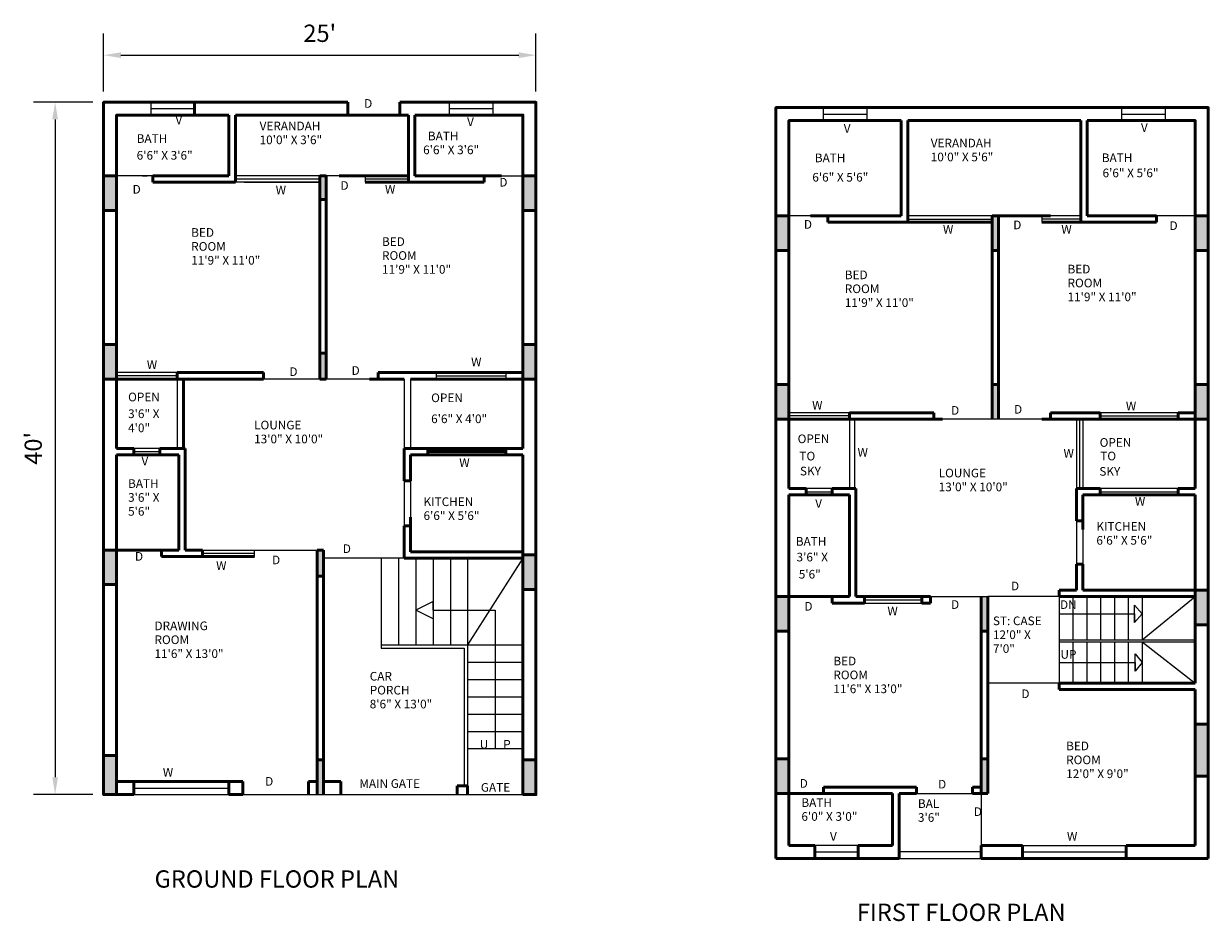
# Model space of a CAD drawing. Units: feet. Extents: x 9.7 to 78.2, y 171.1 to 223.
import ezdxf

# ---------------------------------------------------------------- set-up
doc = ezdxf.new("R2010")
doc.units = ezdxf.units.FT
for name, color, linetype, lineweight in [('A-ANNO-DIMS', 2, 'Continuous', 18), ('A-ANNO-TEXT', 7, 'Continuous', 18), ('A-AREA-IDEN', 3, 'Continuous', 18), ('A-DOOR', 3, 'Continuous', 25), ('A-FLOR-STRS', 6, 'Continuous', 18), ('A-GLAZ', 4, 'Continuous', 25), ('A-WALL', 7, 'Continuous', 50), ('A-WALL-PATT', 8, 'Continuous', 13)]:
    doc.layers.add(name, color=color, linetype=linetype, lineweight=lineweight)
doc.styles.get("Standard").update_dxf_attribs({"font": 'arial.ttf'})
doc.dimstyles.new('ISO-25', dxfattribs={"dimtxt": 1, "dimasz": 1, "dimexe": 1.25, "dimexo": 0.625, "dimtad": 1, "dimtxsty": 'Standard', "dimcen": 2.5, "dimadec": 0, "dimazin": 0, "dimtfac": 1, "dimtmove": 0, "dimatfit": 3, "dimfxl": 1, "dimarcsym": 0})

# ---------------------------------------------------------------- blocks, each defined once
blk = doc.blocks.new('*D1')
at = {"layer": 'A-ANNO-DIMS', "color": 0, "lineweight": -2, "transparency": 16777216}
for p, q in [((14.295, 219.092), (14.295, 222.433)), ((39.295, 219.092), (39.295, 222.433)), ((15.295, 221.183), (38.295, 221.183))]:
    blk.add_line(p, q, dxfattribs=at)
at = {"layer": 'A-ANNO-DIMS', "color": 0, "transparency": 16777216}
for points in [[(15.295, 221.349), (15.295, 221.016), (14.295, 221.183)], [(38.295, 221.349), (38.295, 221.016), (39.295, 221.183)]]:
    blk.add_solid(points, dxfattribs=at)
at = {"layer": 'Defpoints', "color": 0, "transparency": 16777216}
for p in [(39.295, 221.183), (14.295, 218.467), (39.295, 218.467)]:
    blk.add_point(p, dxfattribs=at)
at = {"layer": 'A-ANNO-DIMS', "color": 0, "transparency": 16777216, "insert": (26.795, 222.318), "char_height": 1, "attachment_point": 5}
blk.add_mtext("25'", dxfattribs=at)
blk = doc.blocks.new('*D2')
at = {"layer": 'A-ANNO-DIMS', "color": 0, "lineweight": -2, "transparency": 16777216}
for p, q in [((13.67, 218.467), (10.243, 218.467)), ((11.493, 217.467), (11.493, 179.467)), ((13.67, 178.467), (10.243, 178.467))]:
    blk.add_line(p, q, dxfattribs=at)
at = {"layer": 'A-ANNO-DIMS', "color": 0, "transparency": 16777216}
for points in [[(11.326, 217.467), (11.659, 217.467), (11.493, 218.467)], [(11.326, 179.467), (11.659, 179.467), (11.493, 178.467)]]:
    blk.add_solid(points, dxfattribs=at)
at = {"layer": 'Defpoints', "color": 0, "transparency": 16777216}
for p in [(14.295, 218.467), (11.493, 178.467), (14.295, 178.467)]:
    blk.add_point(p, dxfattribs=at)
at = {"layer": 'A-ANNO-DIMS', "color": 0, "transparency": 16777216, "insert": (10.357, 198.467), "char_height": 1, "attachment_point": 5, "rotation": 90}
blk.add_mtext("40'", dxfattribs=at)
blk = doc.blocks.new('WIN-1500')
for p, q in [((1.5, 0.375), (0, 0.375)), ((0, 0.187), (1.5, 0.187)), ((0, 0), (1.5, 0))]:
    blk.add_line(p, q)
blk = doc.blocks.new('WIN-4500')
for p, q in [((4.5, 0.375), (0, 0.375)), ((0, 0.187), (4.5, 0.187)), ((4.5, 0), (0, 0))]:
    blk.add_line(p, q)

msp = doc.modelspace()

# ---------------------------------------------------------------- hatches: boundary and pattern name
at = {"layer": 'A-WALL-PATT'}
h = msp.add_hatch(color=256, dxfattribs=at)
h.dxf.hatch_style = 1
h.paths.add_polyline_path([(15.045, 214.217), (14.295, 214.217), (14.295, 212.217), (15.045, 212.217)])
h.paths.add_polyline_path([(27.17, 213.842), (27.17, 214.217), (26.795, 214.217), (26.795, 213.842), (26.795, 212.842), (27.17, 212.842)])
h.paths.add_polyline_path([(27.17, 203.967), (26.795, 203.967), (26.795, 202.467), (27.17, 202.467)])
h.paths.add_polyline_path([(39.295, 214.217), (38.545, 214.217), (38.545, 212.217), (39.295, 212.217)])
h.paths.add_polyline_path([(15.045, 204.467), (14.295, 204.467), (14.295, 202.467), (15.045, 202.467)])
h.paths.add_polyline_path([(15.045, 192.592), (14.295, 192.592), (14.295, 190.592), (15.045, 190.592)])
h.paths.add_polyline_path([(27.02, 192.217), (27.02, 192.592), (26.645, 192.592), (26.645, 191.092), (27.02, 191.092)])
h.paths.add_polyline_path([(39.295, 204.467), (38.545, 204.467), (38.545, 202.467), (39.295, 202.467)])
h.paths.add_polyline_path([(39.295, 192.316), (38.545, 192.316), (38.545, 190.316), (39.295, 190.316)])
h.paths.add_polyline_path([(27.02, 180.467), (26.645, 180.467), (26.645, 178.467), (27.02, 178.467)])
h.paths.add_polyline_path([(15.045, 179.217), (15.045, 180.217), (15.045, 180.717), (14.295, 180.717), (14.295, 178.467), (15.045, 178.467)])
h.paths.add_polyline_path([(39.295, 180.467), (38.545, 180.467), (38.545, 178.467), (39.295, 178.467)])
h.paths.add_polyline_path([(53.919, 180.526), (53.169, 180.526), (53.169, 178.526), (53.919, 178.526)])
h.paths.add_polyline_path([(53.919, 189.901), (53.169, 189.901), (53.169, 187.901), (53.919, 187.901)])
h.paths.add_polyline_path([(53.919, 202.151), (53.169, 202.151), (53.169, 200.151), (53.919, 200.151)])
h.paths.add_polyline_path([(53.919, 211.526), (53.919, 211.901), (53.169, 211.901), (53.169, 209.901), (53.919, 209.901)])
h.paths.add_polyline_path([(66.044, 211.901), (65.669, 211.901), (65.669, 209.901), (66.044, 209.901)])
h.paths.add_polyline_path([(66.044, 202.151), (65.669, 202.151), (65.669, 200.151), (66.044, 200.151)])
h.paths.add_polyline_path([(78.169, 211.901), (77.419, 211.901), (77.419, 209.901), (78.169, 209.901)])
h.paths.add_polyline_path([(78.169, 202.151), (77.419, 202.151), (77.419, 200.526), (77.419, 200.151), (78.169, 200.151)])
h.paths.add_polyline_path([(65.419, 189.901), (65.044, 189.901), (65.044, 187.901), (65.419, 187.901)])
h.paths.add_polyline_path([(65.419, 180.526), (65.044, 180.526), (65.044, 178.526), (65.419, 178.526)])
h.paths.add_polyline_path([(78.169, 190.276), (77.419, 190.276), (77.419, 188.276), (78.169, 188.276)])
h.paths.add_polyline_path([(78.169, 181.526), (78.169, 182.526), (77.419, 182.526), (77.419, 179.526), (78.169, 179.526)])

# ---------------------------------------------------------------- linework, layer by layer
at = {"layer": 'A-DOOR'}
for p, q in [((28.42, 217.717), (31.42, 217.717)), ((30.92, 217.717), (31.42, 217.717)), ((17.07, 214.217), (15.045, 214.217)), ((16.545, 214.217), (16.816, 214.217)), ((17.145, 214.217), (17.07, 214.217)), ((29.42, 214.217), (27.17, 214.217)), ((27.92, 214.217), (29.42, 214.217)), ((28.92, 214.217), (29.42, 214.217)), ((37.295, 214.217), (36.295, 214.217)), ((36.295, 214.217), (38.545, 214.217)), ((56.169, 211.901), (53.919, 211.901)), ((55.169, 211.901), (56.169, 211.901)), ((66.044, 211.901), (68.044, 211.901)), ((68.044, 211.901), (68.544, 211.901)), ((77.419, 211.901), (75.169, 211.901)), ((18.545, 202.467), (18.545, 198.467)), ((26.795, 202.467), (23.545, 202.467)), ((30.17, 202.467), (27.17, 202.467)), ((29.67, 202.467), (30.17, 202.467)), ((32.045, 202.467), (32.045, 198.467)), ((65.669, 200.151), (62.294, 200.151)), ((62.794, 200.151), (62.294, 200.151)), ((69.044, 200.151), (65.669, 200.151)), ((68.544, 200.151), (69.044, 200.151)), ((15.145, 192.592), (15.045, 192.592)), ((15.145, 192.592), (17.645, 192.592)), ((23.02, 192.592), (26.645, 192.592)), ((31.67, 192.117), (27.02, 192.117)), ((53.919, 189.901), (56.419, 189.901)), ((62.107, 189.901), (65.419, 189.901)), ((69.544, 189.901), (65.419, 189.901)), ((35.345, 187.117), (35.345, 179.717)), ((35.145, 186.917), (35.145, 179.717)), ((69.544, 184.901), (65.419, 184.901)), ((35.145, 179.717), (35.145, 178.967)), ((35.345, 179.717), (35.345, 178.967)), ((22.345, 178.467), (23.045, 178.467)), ((53.919, 178.526), (55.919, 178.526)), ((65.044, 178.526), (65.044, 175.526)), ((65.044, 175.151), (60.294, 175.151)), ((60.294, 174.776), (65.044, 174.776))]:
    msp.add_line(p, q, dxfattribs=at)
for points in [[(22.345, 178.467), (38.545, 178.467)], [(61.294, 178.526), (64.544, 178.526)]]:
    msp.add_lwpolyline(points, dxfattribs=at)
at = {"layer": 'A-FLOR-STRS'}
for p, q in [((30.345, 192.117), (30.345, 191.117)), ((31.345, 192.117), (31.345, 191.117)), ((32.345, 192.117), (32.345, 191.117)), ((33.345, 192.117), (33.345, 191.117)), ((34.345, 192.117), (34.345, 191.117)), ((35.345, 192.117), (35.345, 191.117)), ((38.545, 192.117), (35.345, 187.117)), ((30.345, 191.117), (30.345, 187.117)), ((31.345, 191.117), (31.345, 187.117)), ((32.345, 191.117), (32.345, 187.117)), ((33.345, 191.117), (33.345, 187.117)), ((34.345, 191.117), (34.345, 187.117)), ((35.345, 191.117), (35.345, 187.117)), ((69.544, 189.901), (69.544, 187.901)), ((70.344, 189.901), (70.344, 187.901)), ((71.144, 189.901), (71.144, 187.901)), ((71.944, 189.901), (71.944, 187.901)), ((72.744, 189.901), (72.744, 187.901)), ((73.544, 189.901), (73.544, 187.901)), ((74.344, 189.901), (74.344, 187.901)), ((74.344, 187.401), (77.419, 189.901)), ((33.345, 189.617), (32.345, 189.117)), ((33.345, 188.617), (32.345, 189.117)), ((33.345, 189.117), (33.345, 189.617)), ((33.345, 189.117), (36.932, 189.117)), ((33.345, 189.117), (33.345, 188.617)), ((33.345, 189.117), (33.345, 188.617)), ((36.932, 189.117), (36.945, 181.117)), ((73.899, 188.401), (73.899, 189.401)), ((73.899, 189.401), (74.344, 188.901)), ((69.544, 188.901), (73.899, 188.901)), ((73.899, 188.901), (73.899, 188.401)), ((74.344, 188.901), (73.899, 188.401)), ((69.544, 187.901), (69.544, 187.401)), ((70.344, 187.901), (70.344, 187.401)), ((71.144, 187.901), (71.144, 187.401)), ((71.944, 187.901), (71.944, 187.401)), ((72.744, 187.901), (72.744, 187.401)), ((73.544, 187.901), (73.544, 187.401)), ((74.344, 187.901), (74.344, 187.401)), ((30.345, 187.117), (35.345, 187.117)), ((30.345, 187.117), (30.345, 186.917)), ((35.345, 187.117), (38.545, 187.117)), ((69.544, 187.401), (77.419, 187.401)), ((69.544, 187.401), (69.544, 187.391)), ((69.544, 187.391), (69.544, 187.291)), ((69.544, 187.291), (77.419, 187.291)), ((69.544, 187.291), (69.544, 184.901)), ((70.344, 187.291), (70.344, 184.901)), ((71.144, 187.291), (71.144, 184.901)), ((71.944, 187.291), (71.944, 184.901)), ((72.744, 187.291), (72.744, 184.901)), ((73.544, 187.291), (73.544, 184.901)), ((74.344, 187.291), (74.344, 184.901)), ((74.344, 187.291), (77.419, 184.901)), ((30.345, 186.917), (35.145, 186.917)), ((73.931, 185.596), (73.931, 186.596)), ((73.931, 186.596), (74.344, 186.096)), ((35.345, 186.117), (38.545, 186.117)), ((69.544, 186.096), (73.931, 186.096)), ((73.931, 186.096), (73.931, 185.596)), ((74.344, 186.096), (73.931, 185.596)), ((35.345, 185.117), (38.545, 185.117)), ((35.345, 184.117), (38.545, 184.117)), ((35.345, 183.117), (38.545, 183.117)), ((35.345, 182.117), (38.545, 182.117)), ((35.345, 181.117), (38.545, 181.117))]:
    msp.add_line(p, q, dxfattribs=at)
at = {"layer": 'A-GLAZ'}
for p, q in [((17.045, 217.717), (17.045, 218.467)), ((17.045, 218.092), (17.045, 218.467)), ((17.045, 218.467), (19.545, 218.467)), ((17.045, 218.092), (19.545, 218.092)), ((19.545, 218.467), (19.545, 217.717)), ((34.295, 217.717), (34.295, 218.467)), ((34.295, 218.467), (36.795, 218.467)), ((34.295, 218.092), (36.795, 218.092)), ((36.795, 218.467), (36.795, 217.717)), ((55.919, 217.401), (55.919, 218.151)), ((55.919, 218.151), (57.919, 218.151)), ((57.919, 218.151), (58.419, 218.151)), ((58.419, 218.151), (58.419, 217.401)), ((73.169, 217.401), (73.169, 218.151)), ((73.169, 218.151), (75.169, 218.151)), ((75.169, 218.151), (75.669, 218.151)), ((75.669, 218.151), (75.669, 217.401)), ((19.545, 217.717), (17.045, 217.717)), ((34.295, 217.717), (36.795, 217.717)), ((55.919, 217.776), (58.419, 217.776)), ((55.919, 217.401), (58.419, 217.401)), ((73.169, 217.776), (75.669, 217.776)), ((73.169, 217.401), (75.669, 217.401)), ((26.795, 214.217), (21.92, 214.217)), ((21.92, 214.029), (26.795, 214.029)), ((26.795, 213.842), (21.92, 213.842)), ((22.432, 213.842), (26.795, 213.842)), ((31.92, 214.217), (29.42, 214.217)), ((29.92, 214.217), (29.42, 214.217)), ((29.42, 214.217), (29.42, 213.842)), ((29.42, 214.029), (31.92, 214.029)), ((29.42, 213.842), (31.92, 213.842)), ((65.669, 211.901), (60.794, 211.901)), ((60.794, 211.713), (65.669, 211.713)), ((70.794, 211.901), (68.544, 211.901)), ((69.044, 211.901), (68.544, 211.901)), ((68.544, 211.901), (68.544, 211.526)), ((70.794, 211.713), (68.544, 211.713)), ((60.794, 211.526), (65.669, 211.526)), ((68.544, 211.526), (70.794, 211.526)), ((18.545, 202.842), (15.045, 202.842)), ((33.545, 202.467), (33.545, 202.842)), ((33.545, 202.842), (37.545, 202.842)), ((37.545, 202.842), (37.545, 202.467)), ((18.545, 202.654), (15.045, 202.654)), ((15.045, 202.467), (18.545, 202.467)), ((31.67, 202.467), (31.67, 198.467)), ((33.545, 202.654), (37.545, 202.654)), ((37.545, 202.467), (33.545, 202.467)), ((57.419, 200.526), (53.919, 200.526)), ((57.419, 200.338), (53.919, 200.338)), ((53.919, 200.151), (57.419, 200.151)), ((57.419, 200.151), (57.419, 196.151)), ((57.719, 200.151), (57.719, 196.151)), ((70.544, 200.151), (70.544, 196.151)), ((70.732, 196.151), (70.732, 200.151)), ((70.919, 200.151), (70.919, 196.151)), ((31.67, 196.592), (31.67, 193.992)), ((32.045, 196.592), (32.045, 193.992)), ((32.045, 194.492), (32.045, 193.992)), ((70.544, 194.276), (70.544, 191.776)), ((70.919, 193.776), (70.919, 194.276)), ((70.919, 194.276), (70.919, 191.776)), ((20.02, 192.592), (23.02, 192.592)), ((23.02, 192.217), (23.02, 192.592)), ((20.02, 192.404), (23.02, 192.404)), ((20.02, 192.217), (23.02, 192.217)), ((58.294, 189.901), (61.607, 189.901)), ((58.294, 189.713), (61.607, 189.713)), ((58.294, 189.526), (61.607, 189.526)), ((16.045, 179.217), (20.045, 179.217)), ((16.045, 178.842), (21.545, 178.842)), ((20.045, 179.217), (21.545, 179.217)), ((57.919, 175.526), (55.419, 175.526)), ((67.419, 175.526), (73.419, 175.526)), ((55.419, 175.151), (57.919, 175.151)), ((55.919, 174.776), (55.419, 174.776)), ((57.919, 174.776), (55.919, 174.776)), ((67.419, 175.153), (73.419, 175.151)), ((69.419, 174.776), (67.419, 174.776)), ((73.419, 174.776), (69.419, 174.776))]:
    msp.add_line(p, q, dxfattribs=at)
msp.add_lwpolyline([(16.045, 178.467), (21.545, 178.467)], dxfattribs=at)
at = {"layer": 'A-WALL'}
for p, q in [((17.045, 218.467), (19.045, 218.467)), ((19.045, 218.467), (19.545, 218.467)), ((19.545, 218.467), (19.545, 217.717)), ((28.42, 218.467), (28.42, 217.717)), ((31.42, 217.717), (31.42, 218.467)), ((58.919, 218.151), (58.419, 218.151)), ((58.419, 218.151), (58.919, 218.151)), ((15.045, 217.717), (19.545, 217.717)), ((15.045, 217.717), (16.045, 217.717)), ((16.045, 217.717), (17.045, 217.717)), ((19.545, 217.717), (21.545, 217.717)), ((21.545, 217.717), (21.545, 214.217)), ((21.92, 217.717), (21.92, 214.217)), ((21.92, 217.717), (28.42, 217.717)), ((31.92, 217.717), (30.92, 217.717)), ((31.42, 217.717), (31.92, 217.717)), ((31.92, 217.717), (31.92, 214.217)), ((32.295, 217.717), (32.295, 214.217)), ((32.295, 217.717), (34.295, 217.717)), ((32.295, 217.717), (32.295, 214.217)), ((32.295, 217.717), (34.295, 217.717)), ((36.795, 217.717), (38.545, 217.717)), ((53.919, 217.401), (60.419, 217.401)), ((53.919, 217.401), (55.919, 217.401)), ((53.919, 217.401), (55.919, 217.401)), ((58.419, 217.401), (60.419, 217.401)), ((60.419, 217.401), (60.419, 211.901)), ((60.794, 217.401), (70.794, 217.401)), ((60.794, 217.401), (60.794, 211.901)), ((60.794, 217.401), (70.794, 217.401)), ((70.794, 217.401), (70.794, 211.901)), ((71.169, 217.401), (77.419, 217.401)), ((71.169, 217.401), (71.169, 211.901)), ((71.169, 217.401), (73.169, 217.401)), ((71.169, 217.401), (73.169, 217.401)), ((75.669, 217.401), (77.419, 217.401)), ((77.419, 217.401), (77.419, 211.901)), ((77.419, 217.401), (77.419, 211.901)), ((77.419, 217.401), (77.419, 211.901)), ((14.295, 212.217), (14.295, 214.217)), ((14.295, 214.217), (15.045, 214.217)), ((15.045, 214.217), (15.045, 213.842)), ((15.045, 214.217), (15.045, 212.217)), ((21.545, 214.217), (17.145, 214.217)), ((17.145, 214.217), (17.145, 213.842)), ((21.545, 213.842), (17.145, 213.842)), ((17.145, 213.842), (21.92, 213.842)), ((21.545, 214.217), (18.358, 214.217)), ((21.92, 214.217), (21.92, 213.842)), ((26.795, 214.217), (26.795, 213.842)), ((27.17, 214.217), (26.795, 214.217)), ((26.795, 213.842), (26.795, 202.842)), ((26.795, 213.842), (26.795, 212.842)), ((27.17, 213.842), (27.17, 214.217)), ((27.17, 213.842), (27.17, 202.842)), ((27.17, 212.842), (27.17, 213.842)), ((29.42, 214.217), (27.92, 214.217)), ((29.42, 214.217), (28.92, 214.217)), ((31.92, 214.217), (29.42, 214.217)), ((29.42, 214.217), (29.92, 214.217)), ((31.92, 213.842), (29.42, 213.842)), ((31.92, 214.217), (31.92, 213.842)), ((31.92, 213.842), (36.295, 213.842)), ((32.295, 214.217), (36.295, 214.217)), ((32.295, 214.217), (37.295, 214.217)), ((32.295, 213.842), (36.295, 213.842)), ((36.295, 214.217), (36.295, 213.842)), ((38.545, 214.217), (38.545, 212.217)), ((39.295, 214.217), (38.545, 214.217)), ((38.545, 213.842), (38.545, 202.842)), ((39.295, 212.217), (39.295, 214.217)), ((26.795, 212.842), (27.17, 212.842)), ((15.045, 212.217), (14.295, 212.217)), ((38.545, 212.217), (39.295, 212.217)), ((53.169, 209.901), (53.169, 211.901)), ((53.169, 211.901), (53.919, 211.901)), ((53.919, 211.901), (53.919, 209.901)), ((57.169, 211.901), (55.169, 211.901)), ((60.419, 211.901), (56.169, 211.901)), ((56.169, 211.901), (56.169, 211.526)), ((60.419, 211.901), (57.169, 211.901)), ((60.794, 211.901), (60.794, 211.526)), ((65.669, 211.901), (65.669, 209.901)), ((68.544, 211.901), (65.669, 211.901)), ((66.044, 209.901), (66.044, 211.901)), ((68.544, 211.901), (69.044, 211.901)), ((70.794, 211.901), (70.794, 211.526)), ((70.794, 211.526), (70.794, 211.713)), ((71.169, 211.901), (74.169, 211.901)), ((75.169, 211.901), (71.169, 211.901)), ((74.169, 211.901), (75.169, 211.901)), ((75.169, 211.901), (75.169, 211.526)), ((77.419, 211.901), (77.419, 209.901)), ((78.169, 211.901), (77.419, 211.901)), ((78.169, 209.901), (78.169, 211.901)), ((60.419, 211.526), (56.169, 211.526)), ((56.169, 211.526), (60.794, 211.526)), ((65.669, 211.526), (60.794, 211.526)), ((65.669, 211.526), (65.669, 200.526)), ((66.044, 211.526), (66.044, 200.526)), ((70.794, 211.526), (68.544, 211.526)), ((70.794, 211.526), (75.169, 211.526)), ((75.169, 211.526), (71.169, 211.526)), ((77.419, 211.526), (77.419, 200.526)), ((53.919, 209.901), (53.169, 209.901)), ((65.669, 209.901), (66.044, 209.901)), ((77.419, 209.901), (78.169, 209.901)), ((15.045, 204.467), (14.295, 204.467)), ((14.295, 204.467), (14.295, 202.467)), ((15.045, 202.467), (15.045, 204.467)), ((26.795, 202.467), (26.795, 204.467)), ((26.795, 204.467), (26.795, 203.467)), ((27.17, 204.467), (27.17, 202.467)), ((38.545, 202.467), (38.545, 204.467)), ((38.545, 204.467), (39.295, 204.467)), ((39.295, 204.467), (39.295, 202.467)), ((26.795, 203.467), (26.795, 203.967)), ((26.795, 203.967), (27.17, 203.967)), ((23.545, 202.842), (18.545, 202.842)), ((18.545, 202.467), (18.545, 202.842)), ((18.545, 202.842), (22.545, 202.842)), ((22.545, 202.842), (23.545, 202.842)), ((23.545, 202.842), (23.545, 202.467)), ((30.17, 202.467), (30.17, 202.842)), ((33.545, 202.842), (30.17, 202.842)), ((38.545, 202.842), (33.545, 202.842)), ((14.295, 202.467), (15.045, 202.467)), ((18.545, 202.467), (15.045, 202.467)), ((18.545, 202.467), (18.92, 202.467)), ((23.545, 202.467), (18.545, 202.467)), ((18.92, 202.467), (18.92, 198.467)), ((27.17, 202.467), (26.795, 202.467)), ((30.17, 202.467), (29.67, 202.467)), ((31.67, 202.467), (30.17, 202.467)), ((31.67, 202.467), (30.17, 202.467)), ((38.545, 202.467), (32.045, 202.467)), ((32.045, 202.467), (33.045, 202.467)), ((33.545, 202.467), (32.045, 202.467)), ((33.045, 202.467), (33.545, 202.467)), ((38.545, 202.467), (37.545, 202.467)), ((39.295, 202.467), (38.545, 202.467)), ((53.919, 202.151), (53.169, 202.151)), ((53.169, 202.151), (53.169, 200.151)), ((53.919, 200.151), (53.919, 202.151)), ((65.669, 200.151), (65.669, 202.151)), ((65.669, 202.151), (66.044, 202.151)), ((66.044, 202.151), (66.044, 200.151)), ((77.419, 200.151), (77.419, 202.151)), ((77.419, 202.151), (78.169, 202.151)), ((78.169, 202.151), (78.169, 200.151)), ((53.169, 200.151), (53.919, 200.151)), ((62.294, 200.151), (53.919, 200.151)), ((62.294, 200.526), (57.419, 200.526)), ((57.419, 200.151), (57.419, 200.526)), ((62.294, 200.526), (57.419, 200.526)), ((57.794, 200.151), (61.794, 200.151)), ((61.794, 200.151), (62.794, 200.151)), ((62.294, 200.151), (62.294, 200.526)), ((70.544, 200.151), (68.544, 200.151)), ((69.044, 200.151), (69.044, 200.526)), ((71.919, 200.526), (69.044, 200.526)), ((70.544, 200.151), (69.044, 200.151)), ((70.919, 200.151), (70.544, 200.151)), ((77.419, 200.151), (70.919, 200.151)), ((70.919, 200.151), (71.919, 200.151)), ((71.919, 200.151), (70.919, 200.151)), ((71.919, 200.151), (71.919, 200.526)), ((77.419, 200.526), (76.419, 200.526)), ((76.419, 200.151), (76.419, 200.526)), ((77.419, 200.151), (76.419, 200.151)), ((77.419, 200.151), (76.419, 200.151)), ((78.169, 200.151), (77.419, 200.151)), ((15.045, 198.467), (16.045, 198.467)), ((16.045, 198.467), (15.045, 198.467)), ((18.545, 198.092), (15.045, 198.092)), ((15.045, 198.092), (16.045, 198.092)), ((16.045, 198.467), (16.045, 198.092)), ((18.545, 198.467), (17.545, 198.467)), ((18.545, 198.467), (17.545, 198.467)), ((17.545, 198.467), (17.545, 198.092)), ((17.545, 198.092), (18.645, 198.092)), ((18.545, 198.467), (19.02, 198.467)), ((18.645, 198.092), (18.645, 192.592)), ((19.02, 198.467), (19.02, 198.092)), ((19.02, 198.092), (19.02, 192.592)), ((31.67, 198.467), (31.67, 198.092)), ((32.045, 198.467), (31.67, 198.467)), ((31.67, 198.092), (31.67, 196.592)), ((32.045, 198.467), (33.045, 198.467)), ((32.045, 198.467), (33.045, 198.467)), ((32.045, 198.092), (38.545, 198.092)), ((32.045, 198.092), (32.045, 196.592)), ((32.045, 198.092), (32.045, 197.092)), ((33.045, 198.092), (32.045, 198.092)), ((33.045, 198.467), (33.045, 198.092)), ((33.045, 198.467), (37.545, 198.467)), ((33.045, 198.279), (37.545, 198.279)), ((37.545, 198.092), (33.045, 198.092)), ((38.545, 198.467), (37.545, 198.467)), ((37.545, 198.467), (37.545, 198.092)), ((37.545, 198.467), (38.545, 198.467)), ((38.545, 198.092), (37.545, 198.092)), ((32.045, 196.592), (31.67, 196.592)), ((32.045, 197.092), (32.045, 196.592)), ((53.919, 196.151), (54.919, 196.151)), ((54.919, 196.151), (53.919, 196.151)), ((54.919, 196.151), (54.919, 195.776)), ((57.419, 196.151), (56.419, 196.151)), ((57.419, 196.151), (56.419, 196.151)), ((56.419, 196.151), (56.419, 195.776)), ((57.419, 196.151), (57.794, 196.151)), ((57.794, 196.151), (57.794, 195.776)), ((70.544, 196.151), (70.544, 195.776)), ((70.919, 196.151), (70.544, 196.151)), ((70.919, 196.151), (71.919, 196.151)), ((70.919, 196.151), (71.919, 196.151)), ((71.919, 196.151), (71.919, 195.776)), ((77.419, 196.151), (76.419, 196.151)), ((76.419, 196.151), (76.419, 195.776)), ((76.419, 196.151), (77.419, 196.151)), ((57.419, 195.776), (53.919, 195.776)), ((53.919, 195.776), (54.919, 195.776)), ((53.919, 182.276), (53.919, 195.276)), ((56.419, 195.776), (57.419, 195.776)), ((57.419, 195.776), (57.419, 190.276)), ((57.794, 195.776), (57.794, 190.276)), ((70.544, 195.776), (70.544, 194.276)), ((70.919, 195.776), (77.419, 195.776)), ((70.919, 195.776), (70.919, 194.276)), ((70.919, 195.776), (70.919, 194.776)), ((71.919, 195.776), (70.919, 195.776)), ((77.419, 195.776), (76.419, 195.776)), ((70.919, 194.776), (70.919, 193.776)), ((32.045, 193.992), (31.67, 193.992)), ((31.67, 193.992), (31.67, 192.492)), ((32.045, 193.492), (32.045, 194.492)), ((32.045, 193.992), (32.045, 192.492)), ((70.919, 194.276), (70.544, 194.276)), ((32.045, 192.492), (32.045, 193.492)), ((14.295, 190.592), (14.295, 192.592)), ((14.295, 192.592), (15.045, 192.592)), ((15.045, 192.592), (15.045, 190.592)), ((18.645, 192.592), (15.145, 192.592)), ((18.645, 192.592), (17.645, 192.592)), ((17.645, 192.592), (17.645, 192.217)), ((17.645, 192.592), (18.645, 192.592)), ((19.02, 192.592), (20.02, 192.592)), ((19.02, 192.592), (20.02, 192.592)), ((20.02, 192.592), (20.02, 192.217)), ((26.645, 192.592), (26.645, 192.217)), ((27.02, 192.592), (26.645, 192.592)), ((26.645, 192.592), (26.645, 190.592)), ((27.02, 192.217), (27.02, 192.592)), ((31.67, 192.492), (31.67, 192.117)), ((32.045, 192.492), (38.545, 192.492)), ((18.645, 192.217), (17.645, 192.217)), ((17.645, 192.217), (20.02, 192.217)), ((20.02, 192.217), (23.02, 192.217)), ((26.645, 192.217), (26.645, 179.217)), ((27.02, 192.217), (27.02, 179.217)), ((31.67, 192.117), (32.045, 192.117)), ((32.045, 192.117), (38.545, 192.117)), ((38.545, 192.316), (39.295, 192.316)), ((38.545, 190.316), (38.545, 192.316)), ((39.295, 192.316), (39.295, 190.316)), ((70.544, 190.276), (70.544, 191.776)), ((70.544, 191.776), (70.919, 191.776)), ((70.544, 191.776), (70.544, 190.276)), ((70.919, 191.776), (70.919, 190.276)), ((15.045, 190.592), (14.295, 190.592)), ((26.645, 190.592), (26.645, 191.092)), ((26.645, 191.092), (27.02, 191.092)), ((39.295, 190.316), (38.545, 190.316)), ((53.169, 187.901), (53.169, 189.901)), ((53.169, 189.901), (53.919, 189.901)), ((57.419, 189.901), (53.919, 189.901)), ((53.919, 189.901), (53.919, 187.901)), ((57.419, 189.901), (56.419, 189.901)), ((56.419, 189.901), (56.419, 189.526)), ((56.419, 189.901), (57.419, 189.901)), ((57.419, 190.276), (57.419, 189.901)), ((57.794, 190.276), (57.794, 189.901)), ((57.794, 189.901), (62.107, 189.901)), ((57.794, 189.901), (58.294, 189.901)), ((58.294, 189.901), (58.294, 189.526)), ((61.607, 189.901), (61.607, 189.526)), ((61.607, 189.901), (62.107, 189.901)), ((62.107, 189.901), (62.107, 189.526)), ((65.044, 187.901), (65.044, 189.901)), ((65.419, 189.901), (65.419, 178.901)), ((65.419, 189.901), (65.419, 187.901)), ((70.544, 190.276), (69.544, 190.276)), ((69.544, 190.276), (69.544, 189.901)), ((69.544, 189.901), (70.919, 189.901)), ((70.919, 190.276), (77.419, 190.276)), ((70.919, 189.901), (77.419, 189.901)), ((77.419, 190.276), (78.169, 190.276)), ((77.419, 190.276), (77.419, 188.276)), ((78.169, 190.276), (78.169, 188.276)), ((56.419, 189.526), (58.294, 189.526)), ((61.607, 189.526), (62.107, 189.526)), ((65.044, 189.526), (65.044, 178.901)), ((53.919, 187.901), (53.169, 187.901)), ((65.419, 187.901), (65.044, 187.901)), ((78.169, 188.276), (77.419, 188.276)), ((78.169, 188.276), (78.169, 187.526)), ((65.419, 184.526), (65.419, 178.526)), ((77.419, 184.901), (69.544, 184.901)), ((69.544, 184.901), (69.544, 184.526)), ((77.419, 184.526), (69.544, 184.526)), ((77.419, 175.526), (77.419, 184.526)), ((78.169, 182.526), (77.419, 182.526)), ((78.169, 181.526), (78.169, 182.526)), ((53.919, 178.901), (53.919, 181.901)), ((77.419, 177.526), (77.419, 181.526)), ((77.419, 181.526), (77.419, 179.526)), ((78.169, 179.526), (78.169, 181.526)), ((15.045, 180.717), (14.295, 180.717)), ((14.295, 180.717), (14.295, 178.467)), ((15.045, 180.217), (15.045, 180.717)), ((15.045, 179.217), (15.045, 180.217)), ((26.645, 178.467), (26.645, 180.467)), ((26.645, 180.467), (27.02, 180.467)), ((27.02, 180.467), (27.02, 178.467)), ((38.545, 178.467), (38.545, 180.467)), ((38.545, 180.467), (39.295, 180.467)), ((53.919, 180.526), (53.169, 180.526)), ((53.169, 180.526), (53.169, 178.526)), ((53.919, 178.526), (53.919, 180.526)), ((65.419, 180.526), (65.044, 180.526)), ((65.044, 180.526), (65.044, 178.526)), ((65.419, 178.526), (65.419, 180.526)), ((77.419, 179.526), (78.169, 179.526)), ((15.045, 178.467), (15.045, 179.217)), ((15.045, 179.217), (16.045, 179.217)), ((16.045, 179.217), (16.045, 178.467)), ((22.045, 179.217), (21.545, 179.217)), ((21.545, 179.217), (21.545, 178.467)), ((21.545, 179.217), (22.345, 179.217)), ((21.545, 179.217), (22.045, 179.217)), ((22.345, 179.217), (22.345, 178.467)), ((26.645, 179.217), (26.145, 179.217)), ((26.145, 179.217), (26.145, 178.467)), ((27.02, 179.217), (28.02, 179.217)), ((28.02, 179.217), (28.02, 178.467)), ((35.345, 178.967), (34.745, 178.967)), ((34.745, 178.967), (34.745, 178.467)), ((35.345, 178.467), (35.345, 178.967)), ((55.919, 178.526), (55.919, 178.901)), ((61.294, 178.526), (61.294, 178.901)), ((65.044, 178.901), (64.544, 178.901)), ((64.544, 178.901), (64.544, 178.526)), ((65.419, 178.526), (65.419, 178.901)), ((77.419, 178.901), (77.419, 175.526)), ((14.295, 178.467), (15.045, 178.467)), ((22.045, 178.467), (22.345, 178.467)), ((35.345, 178.717), (35.345, 178.467)), ((53.169, 175.526), (53.169, 178.526)), ((53.169, 178.526), (53.919, 178.526)), ((53.919, 175.526), (53.919, 178.526)), ((59.919, 178.526), (55.919, 178.526)), ((55.919, 178.526), (59.919, 178.526)), ((59.919, 178.526), (59.919, 175.526)), ((60.294, 178.526), (60.294, 175.526)), ((60.294, 178.526), (61.294, 178.526)), ((65.044, 178.526), (65.419, 178.526)), ((78.169, 174.776), (78.169, 178.151)), ((77.419, 175.526), (77.419, 177.526)), ((53.169, 174.776), (53.169, 175.526)), ((55.419, 175.526), (53.919, 175.526)), ((55.419, 174.776), (55.419, 175.526)), ((59.919, 175.526), (57.919, 175.526)), ((58.919, 175.526), (57.919, 175.526)), ((57.919, 175.526), (57.919, 174.776)), ((59.919, 175.526), (58.919, 175.526)), ((60.294, 175.526), (60.294, 174.776)), ((65.044, 175.526), (67.419, 175.526)), ((67.419, 175.526), (65.044, 175.526)), ((65.044, 175.526), (65.044, 174.776)), ((67.419, 174.776), (67.419, 175.53)), ((77.419, 175.526), (73.419, 175.526)), ((73.419, 175.526), (73.419, 174.776)), ((73.419, 175.526), (77.419, 175.526)), ((53.919, 174.776), (53.169, 174.776)), ((59.919, 174.776), (53.919, 174.776)), ((54.919, 174.776), (55.419, 174.776)), ((55.419, 174.776), (54.919, 174.776)), ((59.919, 174.776), (60.294, 174.776)), ((65.044, 174.776), (78.169, 174.776))]:
    msp.add_line(p, q, dxfattribs=at)
for points in [[(17.045, 218.467), (14.295, 218.467), (14.295, 178.467), (16.045, 178.467)], [(19.545, 218.467), (17.045, 218.467)], [(28.42, 218.467), (19.545, 218.467)], [(34.295, 218.467), (31.42, 218.467)], [(36.795, 218.467), (34.295, 218.467)], [(38.545, 178.467), (39.295, 178.467), (39.295, 218.467), (36.795, 218.467)], [(78.169, 178.151), (78.169, 218.151), (53.169, 218.151), (53.169, 178.151)], [(17.045, 217.717), (15.045, 217.717), (15.045, 214.217)], [(21.545, 217.717), (17.045, 217.717)], [(31.92, 217.717), (21.92, 217.717)], [(38.545, 198.467), (38.545, 217.717), (32.295, 217.717)], [(60.419, 217.401), (53.919, 217.401), (53.919, 211.901)], [(70.794, 217.401), (60.794, 217.401)], [(77.419, 196.151), (77.419, 217.401), (71.169, 217.401)], [(15.045, 213.842), (15.045, 198.467)], [(53.919, 211.526), (53.919, 196.151)], [(15.045, 198.092), (15.045, 179.217), (22.345, 179.217)], [(38.545, 179.217), (38.545, 198.092)], [(53.919, 195.776), (53.919, 178.901)], [(77.419, 190.276), (77.419, 195.776)], [(77.419, 184.901), (77.419, 189.901)], [(77.419, 178.901), (77.419, 184.526)], [(26.145, 179.217), (26.645, 179.217)], [(27.02, 179.217), (28.02, 179.217)], [(55.919, 178.901), (61.294, 178.901)], [(64.544, 178.901), (65.044, 178.901)], [(21.545, 178.467), (22.345, 178.467)], [(53.919, 178.526), (59.919, 178.526)], [(60.294, 178.526), (61.294, 178.526)], [(64.544, 178.526), (65.419, 178.526)]]:
    msp.add_lwpolyline(points, dxfattribs=at)

# ---------------------------------------------------------------- block references
at = {"layer": 'A-GLAZ'}
for name, p in [('WIN-4500', (71.919, 200.151)), ('WIN-1500', (16.045, 198.092)), ('WIN-1500', (54.919, 195.776)), ('WIN-4500', (71.919, 195.776))]:
    msp.add_blockref(name, p, dxfattribs=at)

# ---------------------------------------------------------------- texts
at = {"layer": 'A-ANNO-TEXT'}
for s, height, p in [('D', 0.5, (29.361, 218.141)), ('V', 0.5, (18.45, 217.186)), ('V', 0.5, (35.313, 217.09)), ('V', 0.5, (57.091, 216.703)), ('V', 0.5, (74.274, 216.752)), ('D', 0.5, (27.993, 213.403)), ('D', 0.5, (37.176, 213.593)), ('D', 0.5, (15.971, 213.184)), ('W', 0.5, (24.247, 213.143)), ('W', 0.5, (30.564, 213.189)), ('D', 0.5, (54.787, 211.155)), ('W', 0.5, (62.827, 210.87)), ('D', 0.5, (66.891, 211.124)), ('W', 0.5, (69.671, 210.87)), ('D', 0.5, (75.928, 211.083)), ('W', 0.5, (16.795, 203.056)), ('W', 0.5, (35.545, 203.21)), ('D', 0.5, (25.037, 202.648)), ('D', 0.5, (28.635, 202.714)), ('W', 0.5, (55.262, 200.711)), ('D', 0.5, (63.296, 200.411)), ('D', 0.5, (66.935, 200.473)), ('W', 0.5, (73.403, 200.663)), ('V', 0.5, (16.486, 197.486)), ('W', 0.5, (57.889, 197.988)), ('W', 0.5, (69.798, 197.928)), ('W', 0.5, (34.86, 197.387)), ('V', 0.5, (55.441, 195.031)), ('W', 0.5, (73.926, 195.159)), ('D', 0.5, (16.11, 191.975)), ('D', 0.5, (28.127, 192.421)), ('W', 0.5, (20.802, 191.444)), ('D', 0.5, (24.033, 191.769)), ('D', 0.5, (66.761, 190.264)), ('D', 0.5, (54.815, 189.091)), ('W', 0.5, (59.616, 188.818)), ('D', 0.5, (63.294, 189.194)), ('DN', 0.5, (69.594, 189.189)), ('UP', 0.5, (69.622, 186.313)), ('D', 0.5, (67.359, 184.037)), ('U', 0.5, (36.045, 181.117)), ('P', 0.5, (37.398, 181.117)), ('W', 0.5, (17.721, 179.507)), ('D', 0.5, (23.637, 178.978)), ('MAIN GATE', 0.5, (29.083, 178.853)), ('GATE', 0.5, (36.109, 178.63)), ('D', 0.5, (54.542, 178.86)), ('D', 0.5, (62.543, 178.816)), ('D', 0.5, (64.61, 177.227)), ('V', 0.5, (56.295, 175.795)), ('W', 0.5, (69.998, 175.8)), ('GROUND FLOOR PLAN', 1, (17.243, 173.088)), ('FIRST FLOOR PLAN', 1, (57.851, 171.162))]:
    msp.add_text(s, height=height, dxfattribs=at).set_placement(p)
at = {"layer": 'A-AREA-IDEN'}
for s, p in [('VERANDAH', (23.317, 216.843)), ('BATH', (16.208, 216.114)), ('10\'0" X 3\'6"', (23.317, 216.039)), ('BATH', (33.046, 216.264)), ('6\'6" X 3\'6"', (32.771, 215.461)), ('VERANDAH', (62.122, 215.854)), ('6\'6" X 3\'6"', (16.208, 215.146)), ('BATH', (55.418, 215)), ('10\'0" X 5\'6"', (62.122, 215.05)), ('BATH', (72.011, 215.005)), ('6\'6" X 5\'6"', (55.273, 213.879)), ('6\'6" X 5\'6"', (72.054, 214.129)), ('BED', (19.362, 210.688)), ('ROOM', (19.362, 209.884)), ('BED', (30.393, 210.161)), ('11\'9" X 11\'0"', (19.362, 209.081)), ('ROOM', (30.393, 209.358)), ('11\'9" X 11\'0"', (30.393, 208.555)), ('BED', (70.03, 208.574)), ('BED', (57.152, 208.24)), ('ROOM', (70.03, 207.771)), ('ROOM', (57.152, 207.437)), ('11\'9" X 11\'0"', (57.152, 206.634)), ('11\'9" X 11\'0"', (70.03, 206.968)), ('OPEN', (15.712, 201.183)), ('OPEN', (33.234, 201.137)), ('3\'6" X ', (15.712, 200.217)), ('LOUNGE', (22.999, 199.562)), ('6\'6" X 4\'0"', (33.234, 199.924)), ('4\'0"', (15.712, 199.4)), ('13\'0" X 10\'0"', (22.999, 198.759)), ('OPEN', (54.425, 198.768)), ('OPEN', (71.887, 198.557)), ('TO', (54.527, 197.769)), ('TO', (71.922, 197.774)), ('SKY', (54.56, 196.905)), ('LOUNGE', (62.58, 196.791)), ('SKY', (71.869, 196.886)), ('BATH', (15.712, 196.184)), ('3\'6" X ', (15.712, 195.381)), ('13\'0" X 10\'0"', (62.58, 195.988)), ('KITCHEN', (32.793, 195.133)), ('5\'6"', (15.712, 194.577)), ('6\'6" X 5\'6"', (32.793, 194.33)), ('KITCHEN', (71.698, 193.706)), ('BATH', (54.319, 192.843)), ('6\'6" X 5\'6"', (71.698, 192.903)), ('3\'6" X ', (54.362, 191.936)), ('5\'6"', (54.49, 190.944)), ('DRAWING', (17.239, 187.963)), ('ST: CASE', (65.716, 188.252)), ('12\'0" X ', (65.716, 187.449)), ('ROOM', (17.239, 187.16)), ('7\'0"', (65.716, 186.646)), ('11\'6" X 13\'0"', (17.239, 186.357)), ('BED', (56.49, 185.93)), ('ROOM', (56.49, 185.127)), ('CAR', (29.683, 185.05)), ('PORCH', (29.683, 184.247)), ('11\'6" X 13\'0"', (56.49, 184.324)), ('8\'6" X 13\'0"', (29.683, 183.444)), ('BED', (69.95, 181.024)), ('ROOM', (69.95, 180.22)), ('12\'0" X 9\'0"', (69.95, 179.417)), ('BATH', (54.643, 177.752)), ('BAL', (61.381, 177.694)), ('6\'0" X 3\'0"', (54.643, 176.949)), ('3\'6"', (61.381, 176.891))]:
    msp.add_text(s, height=0.5, dxfattribs=at).set_placement(p)

# ---------------------------------------------------------------- dimensions: what is measured, and where the dimension line sits
at = {"layer": 'A-ANNO-DIMS'}
dim = msp.add_linear_dim(base=(39.295, 221.183), p1=(14.295, 218.467), p2=(39.295, 218.467), text="<>'", dimstyle='ISO-25', override={"dimclrd": 0, "dimclre": 0, "dimclrt": 0}, dxfattribs=at)
dim.commit()
dim.dimension.update_dxf_attribs({"geometry": '*D1', "text_midpoint": (26.795, 222.318)})
dim = msp.add_linear_dim(base=(11.493, 178.467), p1=(14.295, 218.467), p2=(14.295, 178.467), angle=90, text="<>'", dimstyle='ISO-25', override={"dimclrd": 0, "dimclre": 0, "dimclrt": 0}, dxfattribs=at)
dim.commit()
dim.dimension.update_dxf_attribs({"geometry": '*D2', "text_midpoint": (10.357, 198.467)})

doc.saveas('drawing.dxf')
